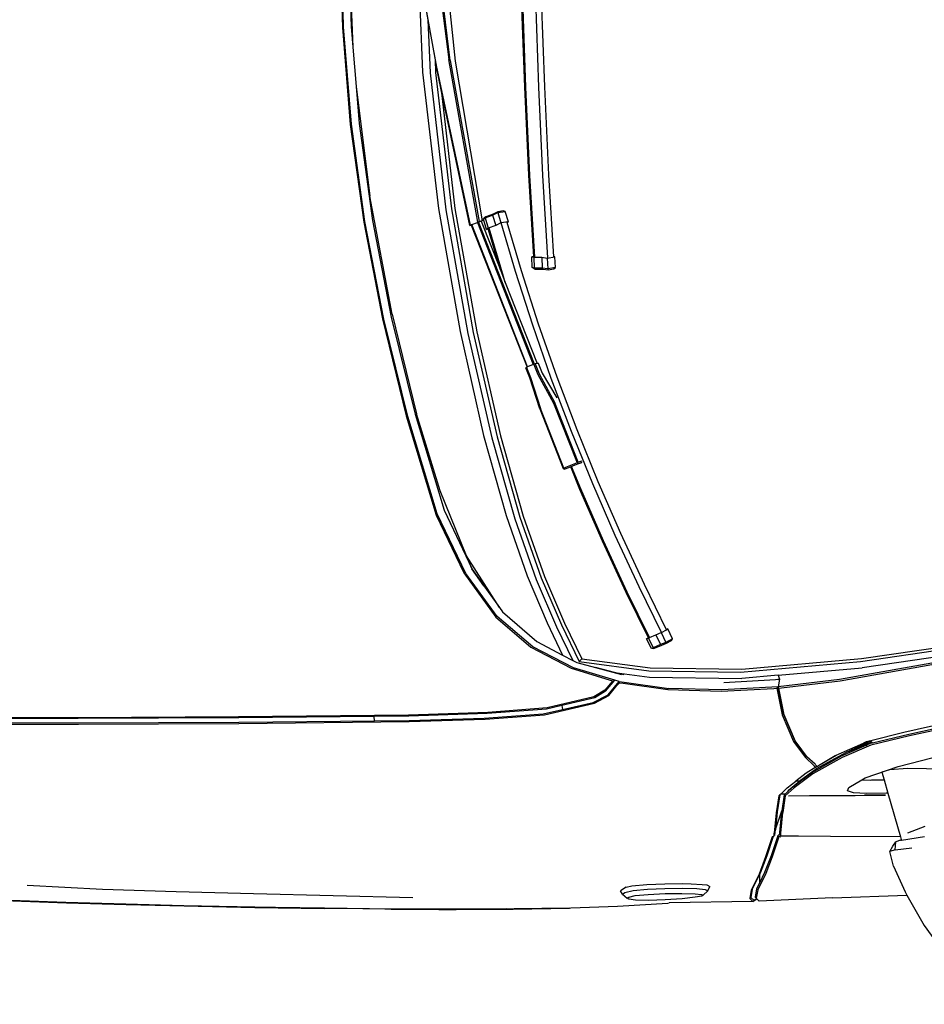
# Model space of a CAD drawing. Units: inches. Extents: x 22042254 to 25404563, y 17568978 to 17626777.
# Tile 2 of 45: x 22042254.4976 to 22042255.0135, y 17568977.6038 to 17568978.1657. Entities that reach past the tile are written whole.
import ezdxf

# ---------------------------------------------------------------- set-up
doc = ezdxf.new("R2010")
doc.units = ezdxf.units.IN
doc.header["$MEASUREMENT"] = 0
doc.layers.add('A-SITE-VEHI', color=8, linetype='Continuous', lineweight=18)
doc.layers.add('Edges', color=250, linetype='Continuous')

# ---------------------------------------------------------------- blocks, each defined once
blk = doc.blocks.new('Nissan Qashqai pl')
at = {"layer": 'Edges'}
for p, q in [((8.8066, 12.84004), (8.85915, 12.91267)), ((8.79082, 12.812), (8.8066, 12.84004)), ((8.19007, 12.82318), (8.1249, 12.82184)), ((8.12514, 12.82198), (8.19016, 12.82331)), ((8.20935, 12.82349), (8.19007, 12.82318)), ((8.19016, 12.82331), (8.25433, 12.82433)), ((8.25433, 12.82433), (8.20935, 12.82349)), ((8.25433, 12.8243), (8.20935, 12.82349)), ((8.25438, 12.8242), (8.20935, 12.82349)), ((8.26926, 12.82449), (8.25433, 12.82433)), ((8.31663, 12.82486), (8.25438, 12.8242)), ((8.31586, 12.82498), (8.26926, 12.82449)), ((8.30977, 12.82497), (8.26926, 12.82449)), ((8.31586, 12.82498), (8.30977, 12.82497)), ((8.31586, 12.82498), (8.31627, 12.82498)), ((8.31627, 12.82498), (8.35975, 12.8252)), ((8.31627, 12.82498), (8.36571, 12.82517)), ((8.37641, 12.82509), (8.31663, 12.82486)), ((8.35975, 12.8252), (8.36571, 12.82517)), ((8.36571, 12.82517), (8.36626, 12.82517)), ((8.36626, 12.82517), (8.3747, 12.8252)), ((8.37641, 12.82509), (8.36626, 12.82517)), ((8.3747, 12.8252), (8.37572, 12.8252)), ((8.37572, 12.8252), (8.4282, 12.82491)), ((8.40688, 12.82493), (8.37641, 12.82509)), ((8.42186, 12.82461), (8.40688, 12.82493)), ((8.42917, 12.82482), (8.40688, 12.82493)), ((8.4282, 12.82491), (8.47991, 12.82391)), ((8.47991, 12.82391), (8.42917, 12.82482)), ((8.47991, 12.82391), (8.48109, 12.82385)), ((8.48109, 12.82385), (8.52408, 12.82218)), ((8.01597, 12.81888), (7.96577, 12.81715)), ((7.96683, 12.81735), (8.01677, 12.81906)), ((8.07131, 12.82051), (8.01597, 12.81888)), ((8.01677, 12.81906), (8.07176, 12.82065)), ((8.1249, 12.82184), (8.07131, 12.82051)), ((8.07176, 12.82065), (8.12514, 12.82198)), ((8.26223, 12.81249), (8.33562, 12.8141)), ((8.52408, 12.82218), (8.5707, 12.81932)), ((8.52871, 12.81123), (8.5331, 12.81495)), ((8.53467, 12.81592), (8.5331, 12.81495)), ((8.5331, 12.81495), (8.53458, 12.81385)), ((8.53458, 12.81385), (8.54056, 12.81253)), ((8.54067, 12.81673), (8.53467, 12.81592)), ((8.55273, 12.81689), (8.54067, 12.81673)), ((8.56822, 12.81638), (8.55273, 12.81689)), ((8.58372, 12.81535), (8.56822, 12.81638)), ((8.5707, 12.81932), (8.57192, 12.81927)), ((8.64892, 12.81786), (8.57192, 12.81927)), ((8.59581, 12.81407), (8.58372, 12.81535)), ((8.6018, 12.81291), (8.59581, 12.81407)), ((8.64602, 12.81526), (8.64604, 12.81528)), ((8.64722, 12.80755), (8.64602, 12.81526)), ((8.64604, 12.81528), (8.64892, 12.81786)), ((8.64703, 12.81416), (8.64984, 12.81684)), ((8.64821, 12.8067), (8.64703, 12.81416)), ((8.64892, 12.81786), (8.65268, 12.81561)), ((8.64984, 12.81684), (8.65238, 12.81531)), ((8.65102, 12.814), (8.65204, 12.81496)), ((8.6524, 12.80636), (8.65102, 12.814)), ((8.65204, 12.81496), (8.65238, 12.81531)), ((8.65344, 12.80726), (8.65204, 12.81496)), ((8.65238, 12.81531), (8.65268, 12.81561)), ((8.65268, 12.81561), (8.65368, 12.81666)), ((8.65469, 12.81761), (8.65368, 12.81666)), ((8.65368, 12.81666), (8.65371, 12.81664)), ((8.7222, 12.8144), (8.65469, 12.81761)), ((8.7222, 12.8144), (8.79082, 12.812)), ((7.98032, 12.80297), (8.04999, 12.80661)), ((8.04999, 12.80661), (8.11758, 12.80867)), ((8.11758, 12.80867), (8.18881, 12.81066)), ((8.18881, 12.81066), (8.26223, 12.81249)), ((8.52871, 12.81123), (8.52689, 12.80817)), ((8.53223, 12.80475), (8.52689, 12.80817)), ((8.52871, 12.81123), (8.53103, 12.80953)), ((8.53103, 12.80953), (8.53854, 12.80786)), ((8.53223, 12.80475), (8.53747, 12.80359)), ((8.53854, 12.80786), (8.55176, 12.80664)), ((8.54056, 12.81253), (8.55262, 12.81139)), ((8.55176, 12.80664), (8.56796, 12.80592)), ((8.55262, 12.81139), (8.5681, 12.81066)), ((8.56796, 12.80592), (8.58417, 12.80574)), ((8.5681, 12.81066), (8.58359, 12.81044)), ((8.58359, 12.81044), (8.59567, 12.81073)), ((8.58417, 12.80574), (8.5974, 12.80608)), ((8.59567, 12.81073), (8.6017, 12.81139)), ((8.5974, 12.80608), (8.60494, 12.8069)), ((8.6017, 12.81139), (8.60325, 12.81209)), ((8.60325, 12.81209), (8.6018, 12.81291)), ((8.60732, 12.80799), (8.60325, 12.81209)), ((8.60494, 12.8069), (8.60732, 12.80799)), ((8.60732, 12.80799), (8.60927, 12.80397)), ((8.65464, 12.79258), (8.64722, 12.80755)), ((8.65502, 12.79287), (8.64821, 12.8067)), ((8.65502, 12.80099), (8.6524, 12.80636)), ((8.66083, 12.7921), (8.65344, 12.80726)), ((8.77849, 12.78548), (8.78905, 12.80886)), ((8.78905, 12.80886), (8.79082, 12.812)), ((8.53747, 12.80359), (8.55126, 12.80232)), ((8.55126, 12.80232), (8.56782, 12.8016)), ((8.56782, 12.8016), (8.58439, 12.80143)), ((8.58439, 12.80143), (8.5921, 12.80163)), ((8.5921, 12.80163), (8.60213, 12.80222)), ((8.60213, 12.80222), (8.6065, 12.80269)), ((8.6065, 12.80269), (8.60927, 12.80397)), ((8.65977, 12.79127), (8.65502, 12.80099)), ((8.65502, 12.79287), (8.65502, 12.80099)), ((8.66062, 12.77679), (8.65464, 12.79258)), ((8.65556, 12.79179), (8.65502, 12.79287)), ((8.65502, 12.79225), (8.65502, 12.79287)), ((8.66163, 12.77582), (8.65556, 12.79179)), ((8.66573, 12.77577), (8.65977, 12.79127)), ((8.66673, 12.77667), (8.66083, 12.7921)), ((8.77849, 12.78548), (8.77507, 12.77189)), ((8.66668, 12.75843), (8.66062, 12.77679)), ((8.66753, 12.75796), (8.66163, 12.77582)), ((8.67178, 12.75741), (8.66573, 12.77577)), ((8.67279, 12.75839), (8.66673, 12.77667)), ((8.77507, 12.77189), (8.7779, 12.76684)), ((8.77984, 12.77027), (8.77507, 12.77189)), ((8.77984, 12.77027), (8.78073, 12.76296)), ((8.77984, 12.77027), (8.7954, 12.76834)), ((8.7779, 12.76684), (8.78073, 12.76296)), ((8.78486, 12.7615), (8.78073, 12.76296)), ((8.78485, 12.75822), (8.7856, 12.7608)), ((8.78486, 12.7615), (8.78581, 12.76135)), ((8.78581, 12.76135), (8.7856, 12.7608)), ((8.78581, 12.76135), (8.80702, 12.75796)), ((8.66753, 12.75796), (8.66668, 12.75843)), ((8.6675, 12.75761), (8.66752, 12.75757)), ((8.66752, 12.75757), (8.66758, 12.75757)), ((8.66786, 12.75779), (8.66753, 12.75796)), ((8.66758, 12.75757), (8.66754, 12.75761)), ((8.66758, 12.75757), (8.66766, 12.75757)), ((8.66766, 12.75757), (8.66765, 12.7576)), ((8.66766, 12.75757), (8.66818, 12.75757)), ((8.66818, 12.75757), (8.66786, 12.75779)), ((8.66818, 12.75757), (8.66923, 12.75661)), ((8.66821, 12.75717), (8.66818, 12.75757)), ((8.66837, 12.75536), (8.66821, 12.75717)), ((8.66821, 12.75717), (8.66923, 12.75661)), ((8.66837, 12.75536), (8.66854, 12.75492)), ((8.6684, 12.755), (8.66837, 12.75536)), ((8.67032, 12.73608), (8.6684, 12.755)), ((8.66923, 12.75661), (8.6697, 12.75191)), ((8.6697, 12.75191), (8.6698, 12.75164)), ((8.67136, 12.73531), (8.6697, 12.75191)), ((8.6698, 12.75164), (8.67553, 12.7343)), ((8.67294, 12.7568), (8.67178, 12.75741)), ((8.67396, 12.7578), (8.67279, 12.75839)), ((8.67326, 12.75663), (8.67294, 12.7568)), ((8.67347, 12.75437), (8.67326, 12.75663)), ((8.67539, 12.73528), (8.67347, 12.75437)), ((8.67424, 12.7576), (8.67396, 12.7578)), ((8.67419, 12.75838), (8.67425, 12.75818)), ((8.67444, 12.75761), (8.67424, 12.7576)), ((8.67443, 12.75503), (8.67424, 12.7576)), ((8.67438, 12.7578), (8.67444, 12.75761)), ((8.67636, 12.736), (8.67443, 12.75503)), ((8.67726, 12.75766), (8.67444, 12.75761)), ((8.67908, 12.7578), (8.677, 12.75781)), ((8.6791, 12.75767), (8.67726, 12.75766)), ((8.72047, 12.75788), (8.67908, 12.7578)), ((8.6791, 12.75767), (8.67908, 12.7578)), ((8.68779, 12.75775), (8.67908, 12.7578)), ((8.68779, 12.75775), (8.6791, 12.75767)), ((8.68779, 12.75775), (8.68781, 12.75771)), ((8.69108, 12.75773), (8.68779, 12.75775)), ((8.72047, 12.75788), (8.69108, 12.75773)), ((8.78485, 12.75822), (8.72047, 12.75788)), ((8.77335, 12.71812), (8.78485, 12.75822)), ((8.79169, 12.7547), (8.80754, 12.74861)), ((8.67268, 12.72067), (8.67032, 12.73608)), ((8.6737, 12.7197), (8.67136, 12.73531)), ((8.67553, 12.7343), (8.67539, 12.73528)), ((8.67775, 12.71956), (8.67553, 12.7343)), ((8.67637, 12.7359), (8.67636, 12.736)), ((8.67876, 12.72047), (8.67637, 12.7359)), ((8.6737, 12.7197), (8.67268, 12.72067)), ((8.67458, 12.71886), (8.6737, 12.7197)), ((8.67852, 12.71886), (8.67458, 12.71886)), ((8.68052, 12.71323), (8.67458, 12.71886)), ((8.67852, 12.71886), (8.67775, 12.71956)), ((8.68152, 12.71616), (8.67852, 12.71886)), ((8.68699, 12.71316), (8.67876, 12.72047)), ((8.68152, 12.71616), (8.68177, 12.7154)), ((8.6817, 12.716), (8.68152, 12.71616)), ((8.6817, 12.716), (8.68177, 12.7154)), ((8.68592, 12.71219), (8.6817, 12.716)), ((8.68177, 12.7204), (8.70119, 12.72032)), ((8.68177, 12.7154), (8.69022, 12.70814)), ((8.70119, 12.72032), (8.70119, 12.72029)), ((8.70119, 12.72032), (8.70264, 12.72028)), ((8.70264, 12.72028), (8.70265, 12.72032)), ((8.70264, 12.72028), (8.70723, 12.72026)), ((8.70723, 12.72026), (8.70724, 12.7203)), ((8.70723, 12.72026), (8.72731, 12.72022)), ((8.72731, 12.72022), (8.7273, 12.72015)), ((8.72731, 12.72022), (8.73541, 12.72019)), ((8.7354, 12.72011), (8.73541, 12.72019)), ((8.73541, 12.72019), (8.74196, 12.72017)), ((8.74149, 12.7177), (8.73614, 12.71582)), ((8.73614, 12.71582), (8.73734, 12.71281)), ((8.75339, 12.71847), (8.74149, 12.7177)), ((8.74196, 12.72007), (8.74196, 12.72017)), ((8.74196, 12.72017), (8.74205, 12.72017)), ((8.74205, 12.72017), (8.74204, 12.72007)), ((8.74205, 12.72017), (8.74259, 12.72016)), ((8.74259, 12.72007), (8.74259, 12.72016)), ((8.74259, 12.72016), (8.74329, 12.72016)), ((8.74329, 12.72006), (8.74329, 12.72016)), ((8.74329, 12.72016), (8.77107, 12.72006)), ((8.77107, 12.72006), (8.75159, 12.72002)), ((8.77184, 12.71812), (8.75339, 12.71847)), ((8.76983, 12.70584), (8.77335, 12.71812)), ((8.77335, 12.71812), (8.77184, 12.71812)), ((8.68052, 12.71323), (8.68839, 12.70708)), ((8.69273, 12.70708), (8.68592, 12.71219)), ((8.70424, 12.7002), (8.68699, 12.71316)), ((8.69166, 12.70708), (8.68839, 12.70708)), ((8.69801, 12.69957), (8.68839, 12.70708)), ((8.69022, 12.70814), (8.69166, 12.70708)), ((8.69166, 12.70708), (8.70745, 12.69546)), ((8.69273, 12.70708), (8.69226, 12.70708)), ((8.70323, 12.69919), (8.69273, 12.70708)), ((8.73734, 12.71281), (8.74923, 12.70589)), ((8.74923, 12.70589), (8.75717, 12.70622)), ((8.74923, 12.70589), (8.75242, 12.70403)), ((8.75717, 12.70622), (8.76983, 12.70584)), ((8.76978, 12.70567), (8.75827, 12.70596)), ((8.76783, 12.69884), (8.76978, 12.70567)), ((8.76978, 12.70567), (8.76983, 12.70584)), ((8.70706, 12.69418), (8.69801, 12.69957)), ((8.73018, 12.68398), (8.70323, 12.69919)), ((8.73122, 12.68505), (8.70424, 12.7002)), ((8.75242, 12.70403), (8.78282, 12.69339)), ((8.77482, 12.6967), (8.76783, 12.69884)), ((8.79161, 12.69538), (8.77482, 12.6967)), ((8.82591, 12.6959), (8.79161, 12.69538)), ((8.69702, 12.685), (8.70548, 12.69273)), ((8.69793, 12.68388), (8.70617, 12.69146)), ((8.70617, 12.69146), (8.69867, 12.68446)), ((8.70548, 12.69273), (8.70706, 12.69418)), ((8.70617, 12.69146), (8.70675, 12.69195)), ((8.70675, 12.69195), (8.70829, 12.6934)), ((8.70706, 12.69418), (8.70829, 12.6934)), ((8.70745, 12.69546), (8.73458, 12.6806)), ((8.70832, 12.69343), (8.70829, 12.6934)), ((8.70832, 12.69338), (8.70829, 12.6934)), ((8.70832, 12.69338), (8.70832, 12.69343)), ((8.71019, 12.69229), (8.70832, 12.69338)), ((8.71021, 12.69228), (8.71019, 12.69229)), ((8.71084, 12.69191), (8.71021, 12.69228)), ((8.72567, 12.68326), (8.71084, 12.69191)), ((8.72477, 12.68364), (8.71084, 12.69191)), ((8.78282, 12.69339), (8.8245, 12.68281)), ((8.68642, 12.6706), (8.69702, 12.685)), ((8.68755, 12.66979), (8.69793, 12.68388)), ((8.69867, 12.68446), (8.69243, 12.67602)), ((8.72567, 12.68326), (8.72477, 12.68364)), ((8.72575, 12.6832), (8.72567, 12.68326)), ((8.72575, 12.6832), (8.75076, 12.67195)), ((8.75292, 12.67414), (8.73018, 12.68398)), ((8.75744, 12.67372), (8.73122, 12.68505)), ((8.73458, 12.6806), (8.74911, 12.67384)), ((8.73458, 12.6806), (8.75774, 12.67094)), ((8.67593, 12.64592), (8.68642, 12.6706)), ((8.67716, 12.64536), (8.68755, 12.66979)), ((8.68828, 12.67043), (8.67767, 12.64575)), ((8.69243, 12.67602), (8.68828, 12.67043)), ((8.69243, 12.67602), (8.69239, 12.67616)), ((8.75076, 12.67195), (8.74911, 12.67384)), ((8.74911, 12.67384), (8.7576, 12.66988)), ((8.75323, 12.67084), (8.75076, 12.67195)), ((8.75292, 12.67414), (8.75774, 12.67094)), ((8.75696, 12.67239), (8.75292, 12.67414)), ((8.75751, 12.66977), (8.75323, 12.67084)), ((8.75874, 12.67197), (8.75696, 12.67239)), ((8.79306, 12.6653), (8.75744, 12.67372)), ((8.7576, 12.66988), (8.75751, 12.66977)), ((8.7881, 12.66207), (8.75751, 12.66977)), ((8.75825, 12.67073), (8.7576, 12.66988)), ((8.75774, 12.67094), (8.75825, 12.67073)), ((8.75901, 12.6717), (8.75825, 12.67073)), ((8.75874, 12.67197), (8.75901, 12.6717)), ((8.75914, 12.67187), (8.75874, 12.67197)), ((8.75914, 12.67187), (8.75901, 12.6717)), ((8.79247, 12.66397), (8.75914, 12.67187)), ((8.89182, 12.63919), (8.7881, 12.66207)), ((8.89406, 12.64182), (8.79247, 12.66397)), ((8.8942, 12.64323), (8.79306, 12.6653)), ((7.90357, 12.65342), (8.0275, 12.6533)), ((7.90396, 12.65472), (8.02759, 12.65454)), ((8.0275, 12.6533), (8.17546, 12.6527)), ((8.02759, 12.65454), (8.17534, 12.65386)), ((8.17534, 12.65386), (8.33243, 12.65213)), ((8.17546, 12.6527), (8.30049, 12.65138)), ((8.30049, 12.65138), (8.30019, 12.64741)), ((8.30049, 12.65138), (8.33242, 12.65104)), ((8.33242, 12.65104), (8.40141, 12.64883)), ((8.33243, 12.65213), (8.40223, 12.64982)), ((8.02732, 12.64849), (7.90142, 12.64867)), ((8.02749, 12.64934), (7.90204, 12.64948)), ((8.17527, 12.64786), (8.02732, 12.64849)), ((8.17541, 12.64873), (8.02749, 12.64934)), ((8.33175, 12.64617), (8.17527, 12.64786)), ((8.30019, 12.64741), (8.17541, 12.64873)), ((8.33197, 12.64707), (8.30019, 12.64741)), ((8.40486, 12.64371), (8.33175, 12.64617)), ((8.40425, 12.64469), (8.33197, 12.64707)), ((8.40141, 12.64883), (8.45586, 12.64505)), ((8.40223, 12.64982), (8.45708, 12.64586)), ((8.45884, 12.64053), (8.40425, 12.64469)), ((8.45947, 12.63948), (8.40486, 12.64371)), ((8.45586, 12.64505), (8.47359, 12.64094)), ((8.45708, 12.64586), (8.50294, 12.635)), ((8.67156, 12.62423), (8.67593, 12.64592)), ((8.67716, 12.64536), (8.6721, 12.62009)), ((8.67767, 12.64575), (8.67272, 12.62129)), ((8.47287, 12.63723), (8.45884, 12.64053)), ((8.50247, 12.62935), (8.45947, 12.63948)), ((8.47287, 12.63723), (8.47359, 12.64094)), ((8.50324, 12.63009), (8.47287, 12.63723)), ((8.47359, 12.64094), (8.50181, 12.6344)), ((8.50181, 12.6344), (8.51552, 12.62739)), ((8.50294, 12.635), (8.51632, 12.62793)), ((8.51253, 12.62314), (8.50247, 12.62935)), ((8.5132, 12.62397), (8.50324, 12.63009)), ((8.51766, 12.61698), (8.51253, 12.62314)), ((8.5132, 12.62397), (8.52164, 12.61386)), ((8.51552, 12.62739), (8.5258, 12.61509)), ((8.51632, 12.62793), (8.52367, 12.61894)), ((8.57063, 12.62256), (8.61967, 12.62406)), ((8.61967, 12.62406), (8.66831, 12.62153)), ((8.67099, 12.62142), (8.67156, 12.62423)), ((8.51661, 12.61349), (8.51971, 12.61447)), ((8.51971, 12.61447), (8.51766, 12.61698)), ((8.51971, 12.61447), (8.52164, 12.61386)), ((8.5258, 12.61509), (8.52164, 12.61386)), ((8.52367, 12.61894), (8.52592, 12.61624)), ((8.52592, 12.61624), (8.5258, 12.61509)), ((8.5258, 12.61509), (8.5304, 12.61573)), ((8.52592, 12.61624), (8.52937, 12.61673)), ((8.52937, 12.61673), (8.57063, 12.62256)), ((8.5304, 12.61573), (8.53043, 12.61574)), ((8.53043, 12.61574), (8.57154, 12.62148)), ((8.62035, 12.62286), (8.57154, 12.62148)), ((8.62035, 12.62286), (8.62038, 12.62286)), ((8.6721, 12.62009), (8.62038, 12.62286)), ((8.62205, 12.61611), (8.66989, 12.61318)), ((8.66831, 12.62153), (8.67099, 12.62142)), ((8.67099, 12.62142), (8.6721, 12.62009)), ((8.67272, 12.62129), (8.6721, 12.62009)), ((8.67332, 12.61285), (8.6721, 12.62009)), ((8.72874, 12.61343), (8.6721, 12.62009)), ((8.67272, 12.62129), (8.67531, 12.621)), ((8.67531, 12.621), (8.72921, 12.61463)), ((8.72921, 12.61463), (8.86656, 12.59005)), ((8.48142, 12.60286), (8.51661, 12.61349)), ((8.52164, 12.61386), (8.48381, 12.60269)), ((8.48894, 12.59687), (8.55313, 12.60545)), ((8.50391, 12.60231), (8.52797, 12.60881)), ((8.52159, 12.60682), (8.50391, 12.60231)), ((8.52159, 12.60682), (8.5538, 12.61113)), ((8.53014, 12.60901), (8.52159, 12.60682)), ((8.55313, 12.60545), (8.6375, 12.60659)), ((8.5538, 12.61113), (8.63869, 12.61228)), ((8.6375, 12.60659), (8.74806, 12.59685)), ((8.6721, 12.60934), (8.63869, 12.61228)), ((8.66989, 12.61318), (8.6721, 12.61297)), ((8.6721, 12.61271), (8.6721, 12.61297)), ((8.6721, 12.61297), (8.67332, 12.61285)), ((8.6721, 12.60934), (8.67332, 12.61285)), ((8.6721, 12.60934), (8.74957, 12.60252)), ((8.86656, 12.58878), (8.72874, 12.61343)), ((8.44441, 12.58341), (8.48142, 12.60286)), ((8.48381, 12.60269), (8.44622, 12.58328)), ((8.47252, 12.56301), (8.48894, 12.59687)), ((8.48305, 12.59574), (8.48667, 12.59765)), ((8.48667, 12.59765), (8.50391, 12.60231)), ((8.49139, 12.59418), (8.48894, 12.59687)), ((8.49139, 12.59418), (8.55442, 12.6026)), ((8.55442, 12.6026), (8.63861, 12.60373)), ((8.63861, 12.60373), (8.74909, 12.59402)), ((8.74806, 12.59685), (8.87447, 12.5782)), ((8.87607, 12.58392), (8.74957, 12.60252)), ((8.44994, 12.57823), (8.47371, 12.5908)), ((8.45936, 12.56105), (8.47371, 12.5908)), ((8.46803, 12.56483), (8.48305, 12.59574)), ((8.47371, 12.5908), (8.48305, 12.59574)), ((8.47556, 12.56152), (8.49139, 12.59418)), ((8.74909, 12.59402), (8.87542, 12.5755)), ((8.41218, 12.55584), (8.44441, 12.58341)), ((8.44622, 12.58328), (8.41339, 12.55539)), ((8.41829, 12.55081), (8.44994, 12.57823)), ((8.5554, 12.58468), (8.55104, 12.57569)), ((8.55286, 12.57507), (8.55721, 12.58406)), ((8.55745, 12.58489), (8.5554, 12.58468)), ((8.55721, 12.58406), (8.5554, 12.58468)), ((8.56386, 12.58101), (8.55721, 12.58406)), ((8.55745, 12.58489), (8.55836, 12.58458)), ((8.55824, 12.58453), (8.55745, 12.58489)), ((8.55836, 12.58458), (8.56493, 12.58156)), ((8.55951, 12.57202), (8.56386, 12.58101)), ((8.56875, 12.57913), (8.56386, 12.58101)), ((8.56439, 12.57013), (8.56875, 12.57913)), ((8.56493, 12.58156), (8.56931, 12.57988)), ((8.56875, 12.57913), (8.56931, 12.57988)), ((8.57488, 12.57575), (8.56875, 12.57913)), ((8.56931, 12.57988), (8.57389, 12.57735)), ((8.55272, 12.57492), (8.53226, 12.53325)), ((8.55368, 12.57469), (8.53316, 12.53288)), ((8.56469, 12.56997), (8.54406, 12.52795)), ((8.55272, 12.57492), (8.55104, 12.57569)), ((8.55104, 12.57569), (8.5528, 12.57509)), ((8.5528, 12.57509), (8.55272, 12.57492)), ((8.5528, 12.57509), (8.55286, 12.57507)), ((8.55286, 12.57507), (8.55368, 12.57469)), ((8.55368, 12.57469), (8.55951, 12.57202)), ((8.55951, 12.57202), (8.56439, 12.57013)), ((8.56439, 12.57013), (8.56469, 12.56997)), ((8.56469, 12.56997), (8.56925, 12.56746)), ((8.57488, 12.57575), (8.57053, 12.56675)), ((8.57389, 12.57735), (8.57488, 12.57575)), ((8.44108, 12.51782), (8.45936, 12.56105)), ((8.44935, 12.52124), (8.46803, 12.56483)), ((8.45396, 12.51963), (8.47252, 12.56301)), ((8.45708, 12.51836), (8.47556, 12.56152)), ((8.54869, 12.52559), (8.5692, 12.56736)), ((8.5692, 12.56736), (8.56925, 12.56746)), ((8.57053, 12.56675), (8.5692, 12.56736)), ((8.56925, 12.56746), (8.57053, 12.56675)), ((8.3826, 12.51507), (8.41218, 12.55584)), ((8.41339, 12.55539), (8.38444, 12.51574)), ((8.41558, 12.54704), (8.41829, 12.55081)), ((8.41545, 12.54683), (8.38521, 12.49936)), ((8.39008, 12.51131), (8.41545, 12.54683)), ((8.40108, 12.52686), (8.41545, 12.54683)), ((8.41558, 12.54704), (8.41545, 12.54683)), ((8.53226, 12.53325), (8.51034, 12.48594)), ((8.53316, 12.53288), (8.51123, 12.48555)), ((8.40108, 12.52686), (8.39008, 12.51131)), ((8.39041, 12.51201), (8.40108, 12.52686)), ((8.54406, 12.52795), (8.52216, 12.48069)), ((8.52689, 12.47854), (8.54869, 12.52559)), ((8.35734, 12.46178), (8.3826, 12.51507)), ((8.38444, 12.51574), (8.3582, 12.46056)), ((8.42173, 12.46216), (8.44108, 12.51782)), ((8.42956, 12.4651), (8.44935, 12.52124)), ((8.43429, 12.46374), (8.45396, 12.51963)), ((8.43748, 12.46269), (8.45708, 12.51836)), ((8.36461, 12.45718), (8.38997, 12.51108)), ((8.36476, 12.45788), (8.38997, 12.51108)), ((8.38997, 12.51108), (8.38521, 12.49936)), ((8.38997, 12.51108), (8.39008, 12.51131)), ((8.39008, 12.51131), (8.39041, 12.51201)), ((8.38521, 12.49936), (8.36083, 12.43935)), ((8.51034, 12.48594), (8.48951, 12.43811)), ((8.51123, 12.48555), (8.49039, 12.4377)), ((8.52216, 12.48069), (8.50136, 12.43291)), ((8.50618, 12.43097), (8.52689, 12.47854)), ((8.32965, 12.37027), (8.35734, 12.46178)), ((8.3582, 12.46056), (8.33108, 12.37081)), ((8.40094, 12.3883), (8.42173, 12.46216)), ((8.40842, 12.39071), (8.42956, 12.4651)), ((8.41325, 12.38959), (8.43429, 12.46374)), ((8.41649, 12.38876), (8.43748, 12.46269)), ((8.33775, 12.36888), (8.36461, 12.45718)), ((8.36461, 12.45718), (8.36475, 12.45786)), ((8.36475, 12.45786), (8.36476, 12.45788)), ((8.36082, 12.43932), (8.33915, 12.3684)), ((8.36082, 12.43932), (8.36083, 12.43935)), ((8.48951, 12.43811), (8.48109, 12.41743)), ((8.50136, 12.43291), (8.48171, 12.38466)), ((8.49039, 12.4377), (8.48199, 12.41707)), ((8.48662, 12.38294), (8.50618, 12.43097)), ((8.45263, 12.36389), (8.47421, 12.41877)), ((8.47475, 12.41851), (8.45317, 12.36363)), ((8.47421, 12.41877), (8.47544, 12.41935)), ((8.47475, 12.41851), (8.47421, 12.41877)), ((8.47544, 12.41935), (8.47475, 12.41851)), ((8.48694, 12.41357), (8.47475, 12.41851)), ((8.47544, 12.41935), (8.48763, 12.4144)), ((8.47906, 12.41826), (8.47544, 12.41935)), ((8.48109, 12.41743), (8.47906, 12.41826)), ((8.48199, 12.41707), (8.48109, 12.41743)), ((8.49125, 12.41331), (8.48199, 12.41707)), ((8.48694, 12.41357), (8.48763, 12.4144)), ((8.48763, 12.4144), (8.49125, 12.41331)), ((8.48763, 12.4144), (8.48814, 12.41311)), ((8.46536, 12.35868), (8.48694, 12.41357)), ((8.48814, 12.41311), (8.46656, 12.35823)), ((8.48814, 12.41311), (8.48694, 12.41357)), ((8.49138, 12.41214), (8.48814, 12.41311)), ((8.49128, 12.41329), (8.49125, 12.41331)), ((8.49128, 12.41322), (8.49128, 12.41329)), ((8.37916, 12.29262), (8.40094, 12.3883)), ((8.38635, 12.29445), (8.40842, 12.39071)), ((8.39129, 12.29354), (8.41325, 12.38959)), ((8.39454, 12.29289), (8.41649, 12.38876)), ((8.48171, 12.38466), (8.46327, 12.33594)), ((8.46826, 12.33445), (8.48662, 12.38294)), ((8.30764, 12.28101), (8.32965, 12.37027)), ((8.33108, 12.37081), (8.3089, 12.28107)), ((8.31566, 12.2795), (8.33775, 12.36888)), ((8.31658, 12.27668), (8.33915, 12.3684)), ((8.45263, 12.36389), (8.44339, 12.33527)), ((8.44394, 12.33502), (8.45317, 12.36363)), ((8.4509, 12.33219), (8.46536, 12.35868)), ((8.4521, 12.33174), (8.46656, 12.35823)), ((8.45473, 12.33095), (8.46822, 12.35383)), ((8.44339, 12.33527), (8.43974, 12.32597)), ((8.44028, 12.32572), (8.44394, 12.33502)), ((8.46327, 12.33594), (8.44609, 12.28682)), ((8.45115, 12.28557), (8.46826, 12.33445)), ((8.38939, 12.19444), (8.44091, 12.32546)), ((8.44147, 12.32523), (8.3899, 12.1941)), ((8.44028, 12.32572), (8.43974, 12.32597)), ((8.44091, 12.32546), (8.44028, 12.32572)), ((8.44147, 12.32523), (8.44091, 12.32546)), ((8.44669, 12.32311), (8.44147, 12.32523)), ((8.44724, 12.32289), (8.4509, 12.33219)), ((8.44844, 12.32244), (8.4521, 12.33174)), ((8.45107, 12.32165), (8.45473, 12.33095)), ((8.39513, 12.19198), (8.44669, 12.32311)), ((8.44788, 12.32265), (8.39633, 12.19153)), ((8.4209, 12.24749), (8.45017, 12.32192)), ((8.44724, 12.32289), (8.44669, 12.32311)), ((8.44788, 12.32265), (8.44724, 12.32289)), ((8.44844, 12.32244), (8.44788, 12.32265)), ((8.45017, 12.32192), (8.44844, 12.32244)), ((8.45107, 12.32165), (8.45017, 12.32192)), ((8.35927, 12.17908), (8.37916, 12.29262)), ((8.36623, 12.1803), (8.38635, 12.29445)), ((8.37126, 12.17963), (8.39129, 12.29354)), ((8.37452, 12.17917), (8.39454, 12.29289)), ((8.29048, 12.19179), (8.30764, 12.28101)), ((8.3089, 12.28107), (8.29164, 12.19132)), ((8.2985, 12.19013), (8.31566, 12.2795)), ((8.44609, 12.28682), (8.43021, 12.23731)), ((8.43534, 12.2363), (8.45115, 12.28557)), ((8.31658, 12.27668), (8.29596, 12.16799)), ((8.41634, 12.23589), (8.4209, 12.24749)), ((8.4209, 12.24749), (8.41908, 12.2418)), ((8.39863, 12.19084), (8.41634, 12.23589)), ((8.41634, 12.23589), (8.40524, 12.19794)), ((8.41908, 12.2418), (8.40606, 12.19727)), ((8.43021, 12.23731), (8.41715, 12.19257)), ((8.42236, 12.19188), (8.43534, 12.2363)), ((8.44571, 12.23369), (8.44521, 12.22375)), ((8.4475, 12.23479), (8.44571, 12.23369)), ((8.44759, 12.23413), (8.44571, 12.23369)), ((8.4471, 12.22419), (8.44759, 12.23413)), ((8.4475, 12.23479), (8.44844, 12.23501)), ((8.45546, 12.23478), (8.4475, 12.23479)), ((8.45487, 12.23412), (8.44759, 12.23413)), ((8.44844, 12.23501), (8.45565, 12.235)), ((8.45438, 12.22418), (8.45487, 12.23412)), ((8.46004, 12.23485), (8.45487, 12.23412)), ((8.45565, 12.235), (8.46028, 12.23565)), ((8.45955, 12.22491), (8.46004, 12.23485)), ((8.46004, 12.23485), (8.46028, 12.23565)), ((8.46706, 12.23366), (8.46004, 12.23485)), ((8.46028, 12.23565), (8.46552, 12.23476)), ((8.46552, 12.23476), (8.46706, 12.23366)), ((8.46706, 12.23366), (8.46657, 12.22372)), ((8.44805, 12.22408), (8.44352, 12.14865)), ((8.44521, 12.22375), (8.4471, 12.22419)), ((8.44707, 12.22387), (8.44706, 12.22375)), ((8.4471, 12.22419), (8.45438, 12.22418)), ((8.45438, 12.22418), (8.45955, 12.22491)), ((8.46007, 12.2247), (8.45551, 12.14879)), ((8.45955, 12.22491), (8.46657, 12.22372)), ((8.46522, 12.22372), (8.46522, 12.22381)), ((8.44706, 12.22375), (8.44255, 12.14854)), ((8.44706, 12.22375), (8.44521, 12.22375)), ((8.46067, 12.1481), (8.46522, 12.22372)), ((8.46657, 12.22372), (8.46522, 12.22372)), ((8.40349, 12.19856), (8.40067, 12.18903)), ((8.40233, 12.18792), (8.40515, 12.19745)), ((8.40515, 12.19745), (8.40349, 12.19856)), ((8.40349, 12.19856), (8.40524, 12.19794)), ((8.41205, 12.19501), (8.40515, 12.19745)), ((8.40524, 12.19794), (8.40521, 12.19782)), ((8.2781, 12.10184), (8.29048, 12.19179)), ((8.29164, 12.19132), (8.27932, 12.10157)), ((8.28622, 12.10078), (8.2985, 12.19013)), ((8.38871, 12.19456), (8.35747, 12.04752)), ((8.38816, 12.19481), (8.36183, 12.06999)), ((8.39567, 12.19173), (8.36877, 12.04191)), ((8.37023, 12.0427), (8.39687, 12.19128)), ((8.37461, 12.04353), (8.3995, 12.19049)), ((8.38871, 12.19456), (8.38816, 12.19481)), ((8.38816, 12.19481), (8.38939, 12.19444)), ((8.38936, 12.19436), (8.38871, 12.19456)), ((8.38936, 12.19436), (8.38939, 12.19444)), ((8.38936, 12.19436), (8.3899, 12.1941)), ((8.3899, 12.1941), (8.39513, 12.19198)), ((8.39513, 12.19198), (8.39633, 12.19153)), ((8.39567, 12.19173), (8.39513, 12.19198)), ((8.39687, 12.19128), (8.39567, 12.19173)), ((8.39633, 12.19153), (8.39863, 12.19084)), ((8.3995, 12.19049), (8.39687, 12.19128)), ((8.3995, 12.19049), (8.39863, 12.19084)), ((8.40067, 12.18903), (8.40233, 12.18792)), ((8.40067, 12.18903), (8.40201, 12.18737)), ((8.40233, 12.18792), (8.40923, 12.18548)), ((8.40923, 12.18548), (8.41205, 12.19501)), ((8.41674, 12.19248), (8.41205, 12.19501)), ((8.41391, 12.18295), (8.41674, 12.19248)), ((8.42371, 12.1914), (8.41674, 12.19248)), ((8.42371, 12.1914), (8.42089, 12.18187)), ((8.42233, 12.19178), (8.42236, 12.19188)), ((8.42236, 12.19188), (8.42371, 12.1914)), ((8.34476, 12.05358), (8.35927, 12.17908)), ((8.35156, 12.05419), (8.36623, 12.1803)), ((8.35665, 12.05382), (8.37126, 12.17963)), ((8.36183, 12.06999), (8.37452, 12.17917)), ((8.40284, 12.18682), (8.40201, 12.18737)), ((8.40201, 12.18737), (8.4027, 12.18713)), ((8.40967, 12.1844), (8.40284, 12.18682)), ((8.40923, 12.18548), (8.41391, 12.18295)), ((8.41386, 12.18214), (8.40967, 12.1844)), ((8.41386, 12.18214), (8.41391, 12.18295)), ((8.41908, 12.18133), (8.41386, 12.18214)), ((8.41391, 12.18295), (8.42089, 12.18187)), ((8.42089, 12.18187), (8.41908, 12.18133)), ((8.2834, 12.06686), (8.29596, 12.16799)), ((8.44255, 12.14854), (8.43872, 12.06738)), ((8.44352, 12.14865), (8.43969, 12.06744)), ((8.45551, 12.14879), (8.45166, 12.06738)), ((8.45684, 12.06694), (8.46067, 12.1481)), ((8.27079, 12.01226), (8.2781, 12.10184)), ((8.27932, 12.10157), (8.27192, 12.01183)), ((8.2834, 12.06686), (8.28622, 12.10078)), ((8.36183, 12.06999), (8.35738, 12.04888)), ((8.28039, 12.03052), (8.2834, 12.06686)), ((8.43872, 12.06738), (8.43593, 11.9861)), ((8.43969, 12.06744), (8.4369, 11.98609)), ((8.45166, 12.06738), (8.44886, 11.98585)), ((8.45405, 11.98566), (8.45684, 12.06694)), ((8.34061, 11.95665), (8.34476, 12.05358)), ((8.34946, 12.00531), (8.35156, 12.05419)), ((8.35615, 12.04214), (8.35665, 12.05382)), ((8.35747, 12.04752), (8.31037, 11.78808)), ((8.37023, 12.0427), (8.33738, 11.78256)), ((8.35615, 12.04214), (8.35738, 12.04888)), ((8.35648, 11.87066), (8.37461, 12.04353)), ((8.33603, 11.78277), (8.36877, 12.04191)), ((8.34946, 12.00531), (8.35615, 12.04214)), ((8.27648, 11.92734), (8.28039, 12.03052)), ((8.27881, 12.01143), (8.28039, 12.03052)), ((8.26824, 11.92208), (8.27079, 12.01226)), ((8.27192, 12.01183), (8.26946, 11.92208)), ((8.27648, 11.92734), (8.27881, 12.01143)), ((8.34061, 11.95665), (8.34946, 12.00531))]:
    blk.add_line(p, q, dxfattribs=at)
blk = doc.blocks.new('CAR')
blk.add_blockref('Nissan Qashqai pl', (-9.74328, -11.91512))

msp = doc.modelspace()

# ---------------------------------------------------------------- block references
at = {"layer": 'A-SITE-VEHI', "xscale": -0.6191396643141144, "yscale": 0.6191396643141144, "zscale": 0.6191396643141144, "rotation": 180}
msp.add_blockref('CAR', (22042255.59333, 17568978.22147), dxfattribs=at)

doc.saveas('drawing.dxf')
